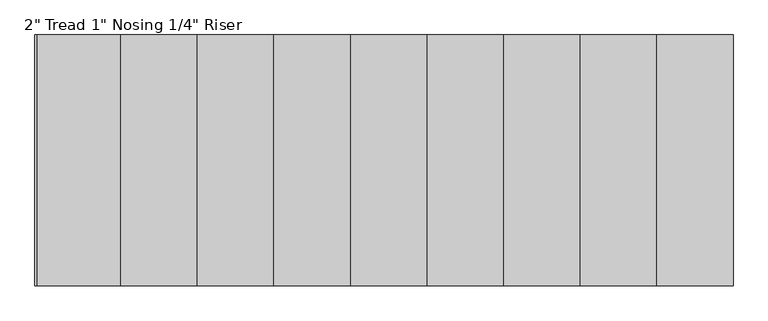
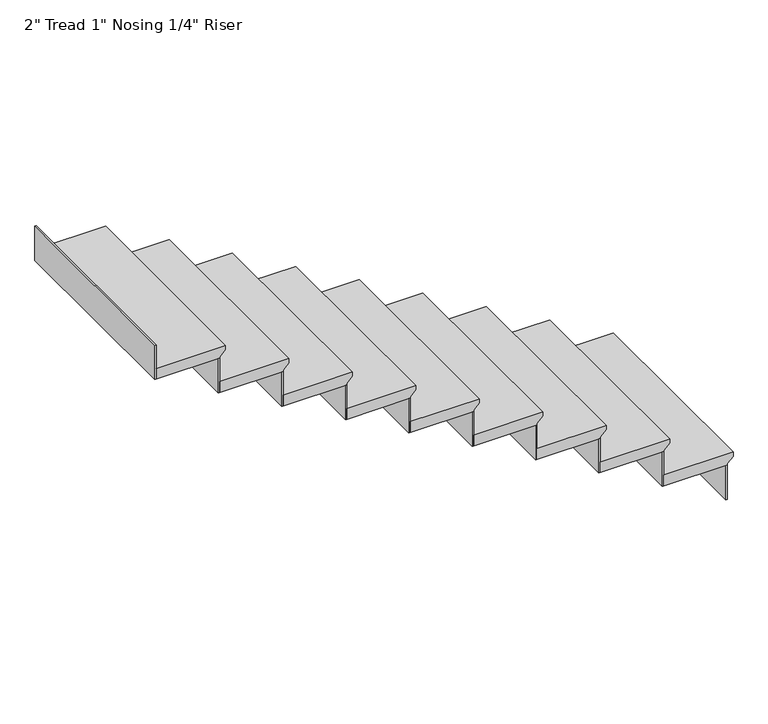
"""IFC4 building model written with IfcOpenShell, lengths in millimetres: stair flight geometry."""

from ifc_helpers import new_model, si_unit, frame, origin, place, context, project, spatial, polyline, outline, extrude, source, transform, mapped, element, save


def stair_flight_de0ef723(model_context):
    return source(origin(), model_context, "Body", "SweptSolid", [
        extrude(outline(polyline([(27363.42, 923.4845537), (27363.42, 618.6845537), (27312.62, 618.6845537), (27312.62, 898.0845537), (27318.97, 898.0845537), (27344.37, 923.4845537), (27363.42, 923.4845537)])), frame((0.0, -5753.3544725, 0.0), z_axis=(0.0, 1.0, 0.0), x_axis=(0.0, 0.0, 1.0)), (0.0, 0.0, 1.0), 914.4),
        extrude(outline(polyline([(891.7345537, -4838.9544725), (898.0845537, -4838.9544725), (898.0845537, -5753.3544725), (891.7345537, -5753.3544725), (891.7345537, -4838.9544725)])), frame((0.0, 0.0, 27152.6), z_axis=(0.0, 0.0, 1.0), x_axis=(1.0, 0.0, 0.0)), (0.0, 0.0, 1.0), 160.02),
        extrude(outline(polyline([(612.3345537, -4838.9544725), (618.6845537, -4838.9544725), (618.6845537, -5753.3544725), (612.3345537, -5753.3544725), (612.3345537, -4838.9544725)])), frame((0.0, 0.0, 27312.62), z_axis=(0.0, 0.0, 1.0), x_axis=(1.0, 0.0, 0.0)), (0.0, 0.0, 1.0), 160.02),
        extrude(outline(polyline([(27523.44, 644.0845537), (27523.44, 339.2845537), (27472.64, 339.2845537), (27472.64, 618.6845537), (27478.99, 618.6845537), (27504.39, 644.0845537), (27523.44, 644.0845537)])), frame((0.0, -5753.3544725, 0.0), z_axis=(0.0, 1.0, 0.0), x_axis=(0.0, 0.0, 1.0)), (0.0, 0.0, 1.0), 914.4),
        extrude(outline(polyline([(332.9345537, -4838.9544725), (339.2845537, -4838.9544725), (339.2845537, -5753.3544725), (332.9345537, -5753.3544725), (332.9345537, -4838.9544725)])), frame((0.0, 0.0, 27472.64), z_axis=(0.0, 0.0, 1.0), x_axis=(1.0, 0.0, 0.0)), (0.0, 0.0, 1.0), 160.02),
        extrude(outline(polyline([(27683.46, 364.6845537), (27683.46, 59.8845537), (27632.66, 59.8845537), (27632.66, 339.2845537), (27639.01, 339.2845537), (27664.41, 364.6845537), (27683.46, 364.6845537)])), frame((0.0, -5753.3544725, 0.0), z_axis=(0.0, 1.0, 0.0), x_axis=(0.0, 0.0, 1.0)), (0.0, 0.0, 1.0), 914.4),
        extrude(outline(polyline([(53.5345537, -4838.9544725), (59.8845537, -4838.9544725), (59.8845537, -5753.3544725), (53.5345537, -5753.3544725), (53.5345537, -4838.9544725)])), frame((0.0, 0.0, 27632.66), z_axis=(0.0, 0.0, 1.0), x_axis=(1.0, 0.0, 0.0)), (0.0, 0.0, 1.0), 160.02),
        extrude(outline(polyline([(27843.48, 85.2845537), (27843.48, -219.5154463), (27792.68, -219.5154463), (27792.68, 59.8845537), (27799.03, 59.8845537), (27824.43, 85.2845537), (27843.48, 85.2845537)])), frame((0.0, -5753.3544725, 0.0), z_axis=(0.0, 1.0, 0.0), x_axis=(0.0, 0.0, 1.0)), (0.0, 0.0, 1.0), 914.4),
        extrude(outline(polyline([(-225.8654463, -4838.9544725), (-219.5154463, -4838.9544725), (-219.5154463, -5753.3544725), (-225.8654463, -5753.3544725), (-225.8654463, -4838.9544725)])), frame((0.0, 0.0, 27792.68), z_axis=(0.0, 0.0, 1.0), x_axis=(1.0, 0.0, 0.0)), (0.0, 0.0, 1.0), 160.02),
        extrude(outline(polyline([(28003.5, -194.1154463), (28003.5, -498.9154463), (27952.7, -498.9154463), (27952.7, -219.5154463), (27959.05, -219.5154463), (27984.45, -194.1154463), (28003.5, -194.1154463)])), frame((0.0, -5753.3544725, 0.0), z_axis=(0.0, 1.0, 0.0), x_axis=(0.0, 0.0, 1.0)), (0.0, 0.0, 1.0), 914.4),
        extrude(outline(polyline([(-505.2654463, -4838.9544725), (-498.9154463, -4838.9544725), (-498.9154463, -5753.3544725), (-505.2654463, -5753.3544725), (-505.2654463, -4838.9544725)])), frame((0.0, 0.0, 27952.7), z_axis=(0.0, 0.0, 1.0), x_axis=(1.0, 0.0, 0.0)), (0.0, 0.0, 1.0), 160.02),
        extrude(outline(polyline([(28163.52, -473.5154463), (28163.52, -778.3154463), (28112.72, -778.3154463), (28112.72, -498.9154463), (28119.07, -498.9154463), (28144.47, -473.5154463), (28163.52, -473.5154463)])), frame((0.0, -5753.3544725, 0.0), z_axis=(0.0, 1.0, 0.0), x_axis=(0.0, 0.0, 1.0)), (0.0, 0.0, 1.0), 914.4),
        extrude(outline(polyline([(-784.6654463, -4838.9544725), (-778.3154463, -4838.9544725), (-778.3154463, -5753.3544725), (-784.6654463, -5753.3544725), (-784.6654463, -4838.9544725)])), frame((0.0, 0.0, 28112.72), z_axis=(0.0, 0.0, 1.0), x_axis=(1.0, 0.0, 0.0)), (0.0, 0.0, 1.0), 160.02),
        extrude(outline(polyline([(28323.54, -752.9154463), (28323.54, -1057.7154463), (28272.74, -1057.7154463), (28272.74, -778.3154463), (28279.09, -778.3154463), (28304.49, -752.9154463), (28323.54, -752.9154463)])), frame((0.0, -5753.3544725, 0.0), z_axis=(0.0, 1.0, 0.0), x_axis=(0.0, 0.0, 1.0)), (0.0, 0.0, 1.0), 914.4),
        extrude(outline(polyline([(-1064.0654463, -4838.9544725), (-1057.7154463, -4838.9544725), (-1057.7154463, -5753.3544725), (-1064.0654463, -5753.3544725), (-1064.0654463, -4838.9544725)])), frame((0.0, 0.0, 28272.74), z_axis=(0.0, 0.0, 1.0), x_axis=(1.0, 0.0, 0.0)), (0.0, 0.0, 1.0), 160.02),
        extrude(outline(polyline([(28483.56, -1032.3154463), (28483.56, -1337.1154463), (28432.76, -1337.1154463), (28432.76, -1057.7154463), (28439.11, -1057.7154463), (28464.51, -1032.3154463), (28483.56, -1032.3154463)])), frame((0.0, -5753.3544725, 0.0), z_axis=(0.0, 1.0, 0.0), x_axis=(0.0, 0.0, 1.0)), (0.0, 0.0, 1.0), 914.4),
        extrude(outline(polyline([(-1343.4654463, -4838.9544725), (-1337.1154463, -4838.9544725), (-1337.1154463, -5753.3544725), (-1343.4654463, -5753.3544725), (-1343.4654463, -4838.9544725)])), frame((0.0, 0.0, 28432.76), z_axis=(0.0, 0.0, 1.0), x_axis=(1.0, 0.0, 0.0)), (0.0, 0.0, 1.0), 160.02),
        extrude(outline(polyline([(-1622.8654463, -4838.9544725), (-1616.5154463, -4838.9544725), (-1616.5154463, -5753.3544725), (-1622.8654463, -5753.3544725), (-1622.8654463, -4838.9544725)])), frame((0.0, 0.0, 28592.78), z_axis=(0.0, 0.0, 1.0), x_axis=(1.0, 0.0, 0.0)), (0.0, 0.0, 1.0), 160.02),
        extrude(outline(polyline([(28643.58, -1311.7154463), (28643.58, -1616.5154463), (28592.78, -1616.5154463), (28592.78, -1337.1154463), (28599.13, -1337.1154463), (28624.53, -1311.7154463), (28643.58, -1311.7154463)])), frame((0.0, -5753.3544725, 0.0), z_axis=(0.0, 1.0, 0.0), x_axis=(0.0, 0.0, 1.0)), (0.0, 0.0, 1.0), 914.4),
    ])


if __name__ == "__main__":
    model = new_model("IFC4")
    model_context = context("Model", 3, world=origin())
    ifc_project = project(units=[si_unit("LENGTHUNIT", "METRE", prefix="MILLI")], contexts=[model_context])
    site = spatial("IfcSite", under=ifc_project)
    building = spatial("IfcBuilding", under=site)
    placement = place(None, origin())
    stair_flight_shape = stair_flight_de0ef723(model_context)
    element("IfcStairFlight", 1, ObjectType="2\" Tread 1\" Nosing 1/4\" Riser", at=placement, inside=building, context=model_context, shape_type="MappedRepresentation", body=[
        mapped(stair_flight_shape, transform((0.0, 0.0, 0.0), x_axis=(1.0, 0.0, 0.0), y_axis=(0.0, 1.0, 0.0), z_axis=(0.0, 0.0, 1.0))),
    ])
    save(model, "model.ifc")
